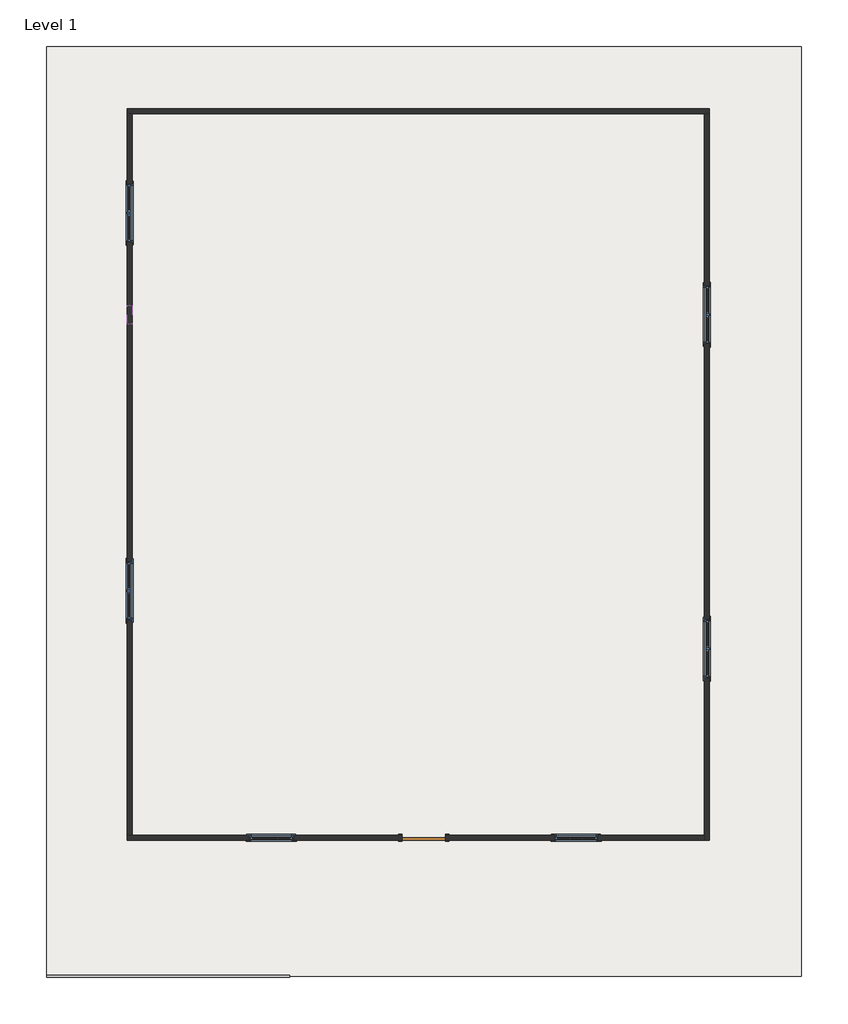
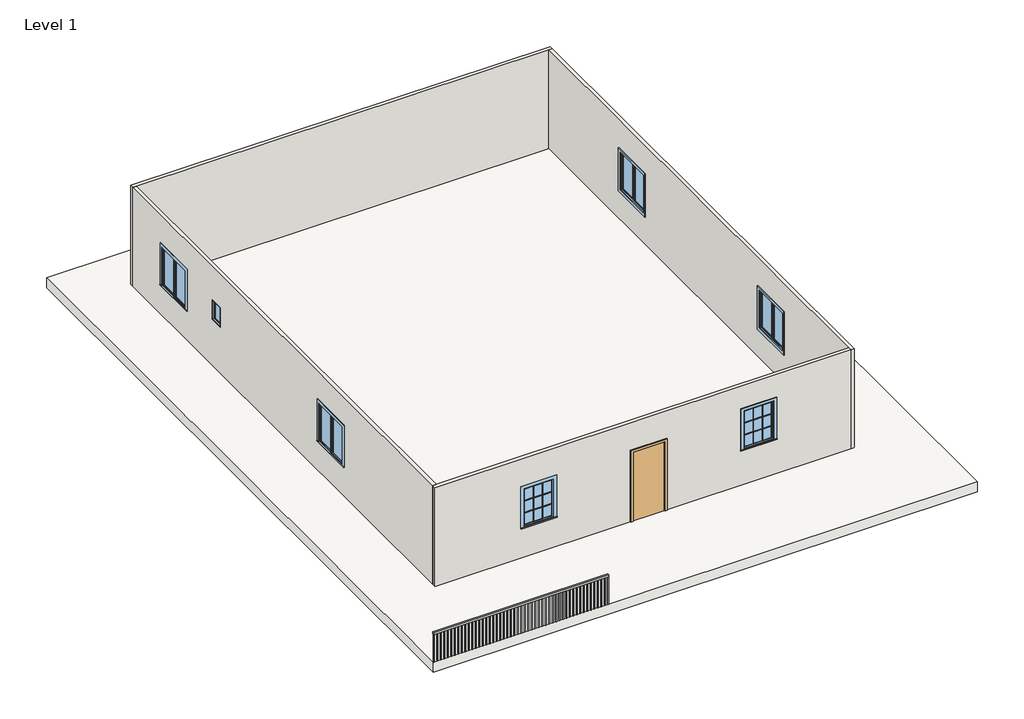
# One storey, incomplete: 7 windows, 4 walls, 1 door, 1 railing, 1 slab.
"""IFC4 building model written with IfcOpenShell, lengths in millimetres."""

from ifc_helpers import new_model, si_unit, frame, origin, origin_with_axes, place, context, project, spatial, polyline, outline, extrude, faceted_brep, transform, mapped, element, save
from components import door_048588e9, window_ad8769eb, window_90ef9153, window_a112695e

model = new_model("IFC4")

# Units and contexts
model_context = context("Model", 3, world=origin())
ifc_project = project(units=[si_unit("LENGTHUNIT", "METRE", prefix="MILLI")], contexts=[model_context])

# Site, building, storey
site = spatial("IfcSite", under=ifc_project)
building = spatial("IfcBuilding", under=site)
storey = spatial("IfcBuildingStorey", under=building, Name="Level 1", Elevation=0.0)

# Door
placement = place(None, origin())
door_shape = door_048588e9(model_context)
element("IfcDoor", 1, ObjectType="Single-Flush : 36\" x 84\"", at=placement, inside=storey, context=model_context, shape_type="MappedRepresentation", body=[
    mapped(door_shape, transform((7992.9168112, -1990.8718204, 0.0), x_axis=(-1.0, 0.0, 0.0), y_axis=(0.0, -1.0, 0.0), z_axis=(0.0, 0.0, 1.0))),
])

# Railing
element("IfcRailing", 2, ObjectType="Handrail - Rectangular", at=placement, inside=storey, context=model_context, shape_type="SweptSolid", body=[
    extrude(outline(polyline([(5173.5168112, -4873.0399729), (5173.5168112, -4923.8399729), (74.1689082, -4923.8399729), (74.1689082, -4873.0399729), (5173.5168112, -4873.0399729)])), frame((0.0, 0.0, 863.6), z_axis=(0.0, 0.0, 1.0), x_axis=(1.0, 0.0, 0.0)), (0.0, 0.0, 1.0), 50.8),
    extrude(outline(polyline([(103.0418112, -4888.9149729), (103.0418112, -4907.9649729), (83.9918112, -4907.9649729), (83.9918112, -4888.9149729), (103.0418112, -4888.9149729)])), origin_with_axes(), (0.0, 0.0, 1.0), 863.6),
    extrude(outline(polyline([(204.6418112, -4888.9149729), (204.6418112, -4907.9649729), (185.5918112, -4907.9649729), (185.5918112, -4888.9149729), (204.6418112, -4888.9149729)])), origin_with_axes(), (0.0, 0.0, 1.0), 863.6),
    extrude(outline(polyline([(306.2418112, -4888.9149729), (306.2418112, -4907.9649729), (287.1918112, -4907.9649729), (287.1918112, -4888.9149729), (306.2418112, -4888.9149729)])), origin_with_axes(), (0.0, 0.0, 1.0), 863.6),
    extrude(outline(polyline([(407.8418112, -4888.9149729), (407.8418112, -4907.9649729), (388.7918112, -4907.9649729), (388.7918112, -4888.9149729), (407.8418112, -4888.9149729)])), origin_with_axes(), (0.0, 0.0, 1.0), 863.6),
    extrude(outline(polyline([(509.4418112, -4888.9149729), (509.4418112, -4907.9649729), (490.3918112, -4907.9649729), (490.3918112, -4888.9149729), (509.4418112, -4888.9149729)])), origin_with_axes(), (0.0, 0.0, 1.0), 863.6),
    extrude(outline(polyline([(611.0418112, -4888.9149729), (611.0418112, -4907.9649729), (591.9918112, -4907.9649729), (591.9918112, -4888.9149729), (611.0418112, -4888.9149729)])), origin_with_axes(), (0.0, 0.0, 1.0), 863.6),
    extrude(outline(polyline([(712.6418112, -4888.9149729), (712.6418112, -4907.9649729), (693.5918112, -4907.9649729), (693.5918112, -4888.9149729), (712.6418112, -4888.9149729)])), origin_with_axes(), (0.0, 0.0, 1.0), 863.6),
    extrude(outline(polyline([(814.2418112, -4888.9149729), (814.2418112, -4907.9649729), (795.1918112, -4907.9649729), (795.1918112, -4888.9149729), (814.2418112, -4888.9149729)])), origin_with_axes(), (0.0, 0.0, 1.0), 863.6),
    extrude(outline(polyline([(915.8418112, -4888.9149729), (915.8418112, -4907.9649729), (896.7918112, -4907.9649729), (896.7918112, -4888.9149729), (915.8418112, -4888.9149729)])), origin_with_axes(), (0.0, 0.0, 1.0), 863.6),
    extrude(outline(polyline([(1017.4418112, -4888.9149729), (1017.4418112, -4907.9649729), (998.3918112, -4907.9649729), (998.3918112, -4888.9149729), (1017.4418112, -4888.9149729)])), origin_with_axes(), (0.0, 0.0, 1.0), 863.6),
    extrude(outline(polyline([(1119.0418112, -4888.9149729), (1119.0418112, -4907.9649729), (1099.9918112, -4907.9649729), (1099.9918112, -4888.9149729), (1119.0418112, -4888.9149729)])), origin_with_axes(), (0.0, 0.0, 1.0), 863.6),
    extrude(outline(polyline([(1220.6418112, -4888.9149729), (1220.6418112, -4907.9649729), (1201.5918112, -4907.9649729), (1201.5918112, -4888.9149729), (1220.6418112, -4888.9149729)])), origin_with_axes(), (0.0, 0.0, 1.0), 863.6),
    extrude(outline(polyline([(1322.2418112, -4888.9149729), (1322.2418112, -4907.9649729), (1303.1918112, -4907.9649729), (1303.1918112, -4888.9149729), (1322.2418112, -4888.9149729)])), origin_with_axes(), (0.0, 0.0, 1.0), 863.6),
    extrude(outline(polyline([(1423.8418112, -4888.9149729), (1423.8418112, -4907.9649729), (1404.7918112, -4907.9649729), (1404.7918112, -4888.9149729), (1423.8418112, -4888.9149729)])), origin_with_axes(), (0.0, 0.0, 1.0), 863.6),
    extrude(outline(polyline([(1525.4418112, -4888.9149729), (1525.4418112, -4907.9649729), (1506.3918112, -4907.9649729), (1506.3918112, -4888.9149729), (1525.4418112, -4888.9149729)])), origin_with_axes(), (0.0, 0.0, 1.0), 863.6),
    extrude(outline(polyline([(1627.0418112, -4888.9149729), (1627.0418112, -4907.9649729), (1607.9918112, -4907.9649729), (1607.9918112, -4888.9149729), (1627.0418112, -4888.9149729)])), origin_with_axes(), (0.0, 0.0, 1.0), 863.6),
    extrude(outline(polyline([(1728.6418112, -4888.9149729), (1728.6418112, -4907.9649729), (1709.5918112, -4907.9649729), (1709.5918112, -4888.9149729), (1728.6418112, -4888.9149729)])), origin_with_axes(), (0.0, 0.0, 1.0), 863.6),
    extrude(outline(polyline([(1830.2418112, -4888.9149729), (1830.2418112, -4907.9649729), (1811.1918112, -4907.9649729), (1811.1918112, -4888.9149729), (1830.2418112, -4888.9149729)])), origin_with_axes(), (0.0, 0.0, 1.0), 863.6),
    extrude(outline(polyline([(1931.8418112, -4888.9149729), (1931.8418112, -4907.9649729), (1912.7918112, -4907.9649729), (1912.7918112, -4888.9149729), (1931.8418112, -4888.9149729)])), origin_with_axes(), (0.0, 0.0, 1.0), 863.6),
    extrude(outline(polyline([(2033.4418112, -4888.9149729), (2033.4418112, -4907.9649729), (2014.3918112, -4907.9649729), (2014.3918112, -4888.9149729), (2033.4418112, -4888.9149729)])), origin_with_axes(), (0.0, 0.0, 1.0), 863.6),
    extrude(outline(polyline([(2135.0418112, -4888.9149729), (2135.0418112, -4907.9649729), (2115.9918112, -4907.9649729), (2115.9918112, -4888.9149729), (2135.0418112, -4888.9149729)])), origin_with_axes(), (0.0, 0.0, 1.0), 863.6),
    extrude(outline(polyline([(2236.6418112, -4888.9149729), (2236.6418112, -4907.9649729), (2217.5918112, -4907.9649729), (2217.5918112, -4888.9149729), (2236.6418112, -4888.9149729)])), origin_with_axes(), (0.0, 0.0, 1.0), 863.6),
    extrude(outline(polyline([(2338.2418112, -4888.9149729), (2338.2418112, -4907.9649729), (2319.1918112, -4907.9649729), (2319.1918112, -4888.9149729), (2338.2418112, -4888.9149729)])), origin_with_axes(), (0.0, 0.0, 1.0), 863.6),
    extrude(outline(polyline([(2439.8418112, -4888.9149729), (2439.8418112, -4907.9649729), (2420.7918112, -4907.9649729), (2420.7918112, -4888.9149729), (2439.8418112, -4888.9149729)])), origin_with_axes(), (0.0, 0.0, 1.0), 863.6),
    extrude(outline(polyline([(2541.4418112, -4888.9149729), (2541.4418112, -4907.9649729), (2522.3918112, -4907.9649729), (2522.3918112, -4888.9149729), (2541.4418112, -4888.9149729)])), origin_with_axes(), (0.0, 0.0, 1.0), 863.6),
    extrude(outline(polyline([(2643.0418112, -4888.9149729), (2643.0418112, -4907.9649729), (2623.9918112, -4907.9649729), (2623.9918112, -4888.9149729), (2643.0418112, -4888.9149729)])), origin_with_axes(), (0.0, 0.0, 1.0), 863.6),
    extrude(outline(polyline([(2744.6418112, -4888.9149729), (2744.6418112, -4907.9649729), (2725.5918112, -4907.9649729), (2725.5918112, -4888.9149729), (2744.6418112, -4888.9149729)])), origin_with_axes(), (0.0, 0.0, 1.0), 863.6),
    extrude(outline(polyline([(2846.2418112, -4888.9149729), (2846.2418112, -4907.9649729), (2827.1918112, -4907.9649729), (2827.1918112, -4888.9149729), (2846.2418112, -4888.9149729)])), origin_with_axes(), (0.0, 0.0, 1.0), 863.6),
    extrude(outline(polyline([(2947.8418112, -4888.9149729), (2947.8418112, -4907.9649729), (2928.7918112, -4907.9649729), (2928.7918112, -4888.9149729), (2947.8418112, -4888.9149729)])), origin_with_axes(), (0.0, 0.0, 1.0), 863.6),
    extrude(outline(polyline([(3049.4418112, -4888.9149729), (3049.4418112, -4907.9649729), (3030.3918112, -4907.9649729), (3030.3918112, -4888.9149729), (3049.4418112, -4888.9149729)])), origin_with_axes(), (0.0, 0.0, 1.0), 863.6),
    extrude(outline(polyline([(3151.0418112, -4888.9149729), (3151.0418112, -4907.9649729), (3131.9918112, -4907.9649729), (3131.9918112, -4888.9149729), (3151.0418112, -4888.9149729)])), origin_with_axes(), (0.0, 0.0, 1.0), 863.6),
    extrude(outline(polyline([(3252.6418112, -4888.9149729), (3252.6418112, -4907.9649729), (3233.5918112, -4907.9649729), (3233.5918112, -4888.9149729), (3252.6418112, -4888.9149729)])), origin_with_axes(), (0.0, 0.0, 1.0), 863.6),
    extrude(outline(polyline([(3354.2418112, -4888.9149729), (3354.2418112, -4907.9649729), (3335.1918112, -4907.9649729), (3335.1918112, -4888.9149729), (3354.2418112, -4888.9149729)])), origin_with_axes(), (0.0, 0.0, 1.0), 863.6),
    extrude(outline(polyline([(3455.8418112, -4888.9149729), (3455.8418112, -4907.9649729), (3436.7918112, -4907.9649729), (3436.7918112, -4888.9149729), (3455.8418112, -4888.9149729)])), origin_with_axes(), (0.0, 0.0, 1.0), 863.6),
    extrude(outline(polyline([(3557.4418112, -4888.9149729), (3557.4418112, -4907.9649729), (3538.3918112, -4907.9649729), (3538.3918112, -4888.9149729), (3557.4418112, -4888.9149729)])), origin_with_axes(), (0.0, 0.0, 1.0), 863.6),
    extrude(outline(polyline([(3659.0418112, -4888.9149729), (3659.0418112, -4907.9649729), (3639.9918112, -4907.9649729), (3639.9918112, -4888.9149729), (3659.0418112, -4888.9149729)])), origin_with_axes(), (0.0, 0.0, 1.0), 863.6),
    extrude(outline(polyline([(3760.6418112, -4888.9149729), (3760.6418112, -4907.9649729), (3741.5918112, -4907.9649729), (3741.5918112, -4888.9149729), (3760.6418112, -4888.9149729)])), origin_with_axes(), (0.0, 0.0, 1.0), 863.6),
    extrude(outline(polyline([(3862.2418112, -4888.9149729), (3862.2418112, -4907.9649729), (3843.1918112, -4907.9649729), (3843.1918112, -4888.9149729), (3862.2418112, -4888.9149729)])), origin_with_axes(), (0.0, 0.0, 1.0), 863.6),
    extrude(outline(polyline([(3963.8418112, -4888.9149729), (3963.8418112, -4907.9649729), (3944.7918112, -4907.9649729), (3944.7918112, -4888.9149729), (3963.8418112, -4888.9149729)])), origin_with_axes(), (0.0, 0.0, 1.0), 863.6),
    extrude(outline(polyline([(4065.4418112, -4888.9149729), (4065.4418112, -4907.9649729), (4046.3918112, -4907.9649729), (4046.3918112, -4888.9149729), (4065.4418112, -4888.9149729)])), origin_with_axes(), (0.0, 0.0, 1.0), 863.6),
    extrude(outline(polyline([(4167.0418112, -4888.9149729), (4167.0418112, -4907.9649729), (4147.9918112, -4907.9649729), (4147.9918112, -4888.9149729), (4167.0418112, -4888.9149729)])), origin_with_axes(), (0.0, 0.0, 1.0), 863.6),
    extrude(outline(polyline([(4268.6418112, -4888.9149729), (4268.6418112, -4907.9649729), (4249.5918112, -4907.9649729), (4249.5918112, -4888.9149729), (4268.6418112, -4888.9149729)])), origin_with_axes(), (0.0, 0.0, 1.0), 863.6),
    extrude(outline(polyline([(4370.2418112, -4888.9149729), (4370.2418112, -4907.9649729), (4351.1918112, -4907.9649729), (4351.1918112, -4888.9149729), (4370.2418112, -4888.9149729)])), origin_with_axes(), (0.0, 0.0, 1.0), 863.6),
    extrude(outline(polyline([(4471.8418112, -4888.9149729), (4471.8418112, -4907.9649729), (4452.7918112, -4907.9649729), (4452.7918112, -4888.9149729), (4471.8418112, -4888.9149729)])), origin_with_axes(), (0.0, 0.0, 1.0), 863.6),
    extrude(outline(polyline([(4573.4418112, -4888.9149729), (4573.4418112, -4907.9649729), (4554.3918112, -4907.9649729), (4554.3918112, -4888.9149729), (4573.4418112, -4888.9149729)])), origin_with_axes(), (0.0, 0.0, 1.0), 863.6),
    extrude(outline(polyline([(4675.0418112, -4888.9149729), (4675.0418112, -4907.9649729), (4655.9918112, -4907.9649729), (4655.9918112, -4888.9149729), (4675.0418112, -4888.9149729)])), origin_with_axes(), (0.0, 0.0, 1.0), 863.6),
    extrude(outline(polyline([(4776.6418112, -4888.9149729), (4776.6418112, -4907.9649729), (4757.5918112, -4907.9649729), (4757.5918112, -4888.9149729), (4776.6418112, -4888.9149729)])), origin_with_axes(), (0.0, 0.0, 1.0), 863.6),
    extrude(outline(polyline([(4878.2418112, -4888.9149729), (4878.2418112, -4907.9649729), (4859.1918112, -4907.9649729), (4859.1918112, -4888.9149729), (4878.2418112, -4888.9149729)])), origin_with_axes(), (0.0, 0.0, 1.0), 863.6),
    extrude(outline(polyline([(4979.8418112, -4888.9149729), (4979.8418112, -4907.9649729), (4960.7918112, -4907.9649729), (4960.7918112, -4888.9149729), (4979.8418112, -4888.9149729)])), origin_with_axes(), (0.0, 0.0, 1.0), 863.6),
    extrude(outline(polyline([(5081.4418112, -4888.9149729), (5081.4418112, -4907.9649729), (5062.3918112, -4907.9649729), (5062.3918112, -4888.9149729), (5081.4418112, -4888.9149729)])), origin_with_axes(), (0.0, 0.0, 1.0), 863.6),
    extrude(outline(polyline([(93.2189082, -4888.9149729), (93.2189082, -4907.9649729), (74.1689082, -4907.9649729), (74.1689082, -4888.9149729), (93.2189082, -4888.9149729)])), origin_with_axes(), (0.0, 0.0, 1.0), 863.6),
    extrude(outline(polyline([(5173.5168112, -4888.9149729), (5173.5168112, -4907.9649729), (5154.4668112, -4907.9649729), (5154.4668112, -4888.9149729), (5173.5168112, -4888.9149729)])), origin_with_axes(), (0.0, 0.0, 1.0), 863.6),
])

# Slab
element("IfcSlab", 3, ObjectType="Generic - 12\"", at=placement, inside=storey, context=model_context, shape_type="SweptSolid", body=[
    extrude(outline(polyline([(15923.7689082, 14608.7600271), (15923.7689082, -4898.4399729), (74.1689082, -4898.4399729), (74.1689082, 14608.7600271), (15923.7689082, 14608.7600271)])), frame((0.0, 0.0, -304.8), z_axis=(0.0, 0.0, 1.0), x_axis=(1.0, 0.0, 0.0)), (0.0, 0.0, 1.0), 304.8),
])

# Walls
element("IfcWall", 4, ObjectType="Generic - 4\" Brick", at=placement, inside=storey, context=model_context, shape_type="Brep", body=[
    faceted_brep([(1769.9168112, 13198.3281796, 0.0), (1871.5168112, 13198.3281796, 0.0), (13885.7168112, 13198.3281796, 0.0), (13987.3168112, 13198.3281796, 0.0), (13987.3168112, 13198.3281796, 3048.0), (13885.7168112, 13198.3281796, 3048.0), (1871.5168112, 13198.3281796, 3048.0), (1769.9168112, 13198.3281796, 3048.0), (1769.9168112, 13299.9281796, 0.0), (1769.9168112, 13299.9281796, 3048.0), (13987.3168112, 13299.9281796, 3048.0), (13987.3168112, 13299.9281796, 0.0)], [[[0, 1, 2, 3, 4, 5, 6, 7]], [[8, 9, 10, 11]], [[3, 2, 1, 0, 8, 11]], [[4, 3, 11, 10]], [[0, 7, 9, 8]], [[7, 6, 5, 4, 10, 9]]]),
])
element("IfcWall", 5, ObjectType="Generic - 4\" Brick", at=placement, inside=storey, context=model_context, shape_type="Brep", body=[
    faceted_brep([(13885.7168112, 13198.3281796, 0.0), (13885.7168112, -1940.0718204, 0.0), (13885.7168112, -2041.6718204, 0.0), (13885.7168112, -2041.6718204, 3048.0), (13885.7168112, -1940.0718204, 3048.0), (13885.7168112, 13198.3281796, 3048.0), (13885.7168112, 1361.9281796, 2133.6), (13885.7168112, 1361.9281796, 914.4), (13885.7168112, 2581.1281796, 914.4), (13885.7168112, 2581.1281796, 2133.6), (13885.7168112, 8372.3281796, 2133.6), (13885.7168112, 8372.3281796, 914.4), (13885.7168112, 9591.5281796, 914.4), (13885.7168112, 9591.5281796, 2133.6), (13987.3168112, 13198.3281796, 0.0), (13987.3168112, 13198.3281796, 3048.0), (13987.3168112, -2041.6718204, 3048.0), (13987.3168112, -2041.6718204, 0.0), (13987.3168112, 1361.9281796, 2133.6), (13987.3168112, 2581.1281796, 2133.6), (13987.3168112, 2581.1281796, 914.4), (13987.3168112, 1361.9281796, 914.4), (13987.3168112, 8372.3281796, 2133.6), (13987.3168112, 9591.5281796, 2133.6), (13987.3168112, 9591.5281796, 914.4), (13987.3168112, 8372.3281796, 914.4)], [[[0, 1, 2, 3, 4, 5], [6, 7, 8, 9], [10, 11, 12, 13]], [[14, 15, 16, 17], [18, 19, 20, 21], [22, 23, 24, 25]], [[2, 1, 0, 14, 17]], [[0, 5, 15, 14]], [[5, 4, 3, 16, 15]], [[3, 2, 17, 16]], [[7, 6, 18, 21]], [[8, 7, 21, 20]], [[9, 8, 20, 19]], [[6, 9, 19, 18]], [[11, 10, 22, 25]], [[12, 11, 25, 24]], [[13, 12, 24, 23]], [[10, 13, 23, 22]]]),
])
element("IfcWall", 6, ObjectType="Generic - 4\" Brick", at=placement, inside=storey, context=model_context, shape_type="Brep", body=[
    faceted_brep([(7535.7168112, -1940.0718204, 2133.6), (7535.7168112, -1940.0718204, 0.0), (1871.5168112, -1940.0718204, 0.0), (1769.9168112, -1940.0718204, 0.0), (1769.9168112, -1940.0718204, 3048.0), (1871.5168112, -1940.0718204, 3048.0), (13885.7168112, -1940.0718204, 3048.0), (13885.7168112, -1940.0718204, 0.0), (8450.1168112, -1940.0718204, 0.0), (8450.1168112, -1940.0718204, 2133.6), (10736.1168112, -1940.0718204, 2288.7570446), (10736.1168112, -1940.0718204, 1069.5570446), (11650.5168112, -1940.0718204, 1069.5570446), (11650.5168112, -1940.0718204, 2288.7570446), (4335.3168112, -1940.0718204, 2133.6), (4335.3168112, -1940.0718204, 914.4), (5249.7168112, -1940.0718204, 914.4), (5249.7168112, -1940.0718204, 2133.6), (1769.9168112, -2041.6718204, 0.0), (7535.7168112, -2041.6718204, 0.0), (7535.7168112, -2041.6718204, 2133.6), (8450.1168112, -2041.6718204, 2133.6), (8450.1168112, -2041.6718204, 0.0), (13885.7168112, -2041.6718204, 0.0), (13885.7168112, -2041.6718204, 3048.0), (1769.9168112, -2041.6718204, 3048.0), (10736.1168112, -2041.6718204, 2288.7570446), (11650.5168112, -2041.6718204, 2288.7570446), (11650.5168112, -2041.6718204, 1069.5570446), (10736.1168112, -2041.6718204, 1069.5570446), (4335.3168112, -2041.6718204, 2133.6), (5249.7168112, -2041.6718204, 2133.6), (5249.7168112, -2041.6718204, 914.4), (4335.3168112, -2041.6718204, 914.4)], [[[0, 1, 2, 3, 4, 5, 6, 7, 8, 9], [10, 11, 12, 13], [14, 15, 16, 17]], [[18, 19, 20, 21, 22, 23, 24, 25], [26, 27, 28, 29], [30, 31, 32, 33]], [[8, 7, 23, 22]], [[3, 2, 1, 19, 18]], [[6, 5, 4, 25, 24]], [[4, 3, 18, 25]], [[7, 6, 24, 23]], [[20, 19, 1, 0]], [[21, 20, 0, 9]], [[22, 21, 9, 8]], [[11, 10, 26, 29]], [[12, 11, 29, 28]], [[13, 12, 28, 27]], [[10, 13, 27, 26]], [[15, 14, 30, 33]], [[16, 15, 33, 32]], [[17, 16, 32, 31]], [[14, 17, 31, 30]]]),
])
element("IfcWall", 7, ObjectType="Generic - 4\" Brick", at=placement, inside=storey, context=model_context, shape_type="SweptSolid", body=[
    extrude(outline(polyline([(13198.3281796, 0.0), (-1940.0718204, 0.0), (-1940.0718204, 3048.0), (13198.3281796, 3048.0), (13198.3281796, 0.0)]), holes=[polyline([(8778.7281796, 2030.6539964), (8778.7281796, 1421.0539964), (9185.1281796, 1421.0539964), (9185.1281796, 2030.6539964), (8778.7281796, 2030.6539964)]), polyline([(11725.1281796, 914.4), (11725.1281796, 2133.6), (10505.9281796, 2133.6), (10505.9281796, 914.4), (11725.1281796, 914.4)]), polyline([(3800.3281796, 914.4), (3800.3281796, 2133.6), (2581.1281796, 2133.6), (2581.1281796, 914.4), (3800.3281796, 914.4)])]), frame((1769.9168112, 0.0, 0.0), z_axis=(1.0, 0.0, 0.0), x_axis=(0.0, 1.0, 0.0)), (0.0, 0.0, 1.0), 101.6),
])

# Windows
window_shape = window_ad8769eb(model_context)
element("IfcWindow", 8, ObjectType="Casement 3x3 with Trim : 36\" x 48\"", at=placement, inside=storey, context=model_context, shape_type="MappedRepresentation", body=[
    mapped(window_shape, transform((11193.3168112, -1990.8718204, 155.1570446), x_axis=(-1.0, 0.0, 0.0), y_axis=(0.0, -1.0, 0.0), z_axis=(0.0, 0.0, 1.0))),
])
element("IfcWindow", 9, ObjectType="Casement 3x3 with Trim : 36\" x 48\"", at=placement, inside=storey, context=model_context, shape_type="MappedRepresentation", body=[
    mapped(window_shape, transform((4792.5168112, -1990.8718204, 0.0), x_axis=(-1.0, 0.0, 0.0), y_axis=(0.0, -1.0, 0.0), z_axis=(0.0, 0.0, 1.0))),
])
window_2_shape = window_90ef9153(model_context)
element("IfcWindow", 10, ObjectType="Casement Dbl with Trim : 48\" x 48\"", at=placement, inside=storey, context=model_context, shape_type="MappedRepresentation", body=[
    mapped(window_2_shape, transform((1839.7668112, 11115.5281796, 0.0), x_axis=(0.0, 1.0, 0.0), y_axis=(-1.0, 0.0, 0.0), z_axis=(0.0, 0.0, 1.0))),
])
element("IfcWindow", 11, ObjectType="Casement Dbl with Trim : 48\" x 48\"", at=placement, inside=storey, context=model_context, shape_type="MappedRepresentation", body=[
    mapped(window_2_shape, transform((1839.7668112, 3190.7281796, 0.0), x_axis=(0.0, 1.0, 0.0), y_axis=(-1.0, 0.0, 0.0), z_axis=(0.0, 0.0, 1.0))),
])
element("IfcWindow", 12, ObjectType="Casement Dbl with Trim : 48\" x 48\"", at=placement, inside=storey, context=model_context, shape_type="MappedRepresentation", body=[
    mapped(window_2_shape, transform((13917.4668112, 1971.5281796, 0.0), x_axis=(0.0, -1.0, 0.0), y_axis=(1.0, 0.0, 0.0), z_axis=(0.0, 0.0, 1.0))),
])
element("IfcWindow", 13, ObjectType="Casement Dbl with Trim : 48\" x 48\"", at=placement, inside=storey, context=model_context, shape_type="MappedRepresentation", body=[
    mapped(window_2_shape, transform((13917.4668112, 8981.9281796, 0.0), x_axis=(0.0, -1.0, 0.0), y_axis=(1.0, 0.0, 0.0), z_axis=(0.0, 0.0, 1.0))),
])
window_3_shape = window_a112695e(model_context)
element("IfcWindow", 14, ObjectType="Fixed : 16\" x 24\"", at=placement, inside=storey, context=model_context, shape_type="MappedRepresentation", body=[
    mapped(window_3_shape, transform((1820.7168112, 8943.8281796, 506.6539964), x_axis=(0.0, -1.0, 0.0), y_axis=(1.0, 0.0, 0.0), z_axis=(0.0, 0.0, 1.0))),
])

save(model, "model.ifc")

# Revit data of these elements
# Type "Single-Flush : 36\" x 84\""
#   Type Mark = "1"
#   Construction Type Id = "MDOOR"
#   Assembly Code = "C1020"
#   Analytic Construction = "Metal"
#   Thickness = 0' - 2"
#   Heat Transfer Coefficient (U) = 0.651978 BTU/(h·ft²·°F)
#   Height = 7' - 0"
#   Trim Projection Ext = 0' - 1"
#   Trim Projection Int = 0' - 1"
#   Trim Width = 0' - 3"
#   Width = 3' - 0"
#   Define Thermal Properties by = 1
#   Door Material = Door - Panel
#   Frame Material = Door - Frame
#   Visual Light Transmittance = 0
#   Solar Heat Gain Coefficient = 0
#   Function = (empty or 0)
#   Wall Closure = (empty or 0)
# Type "Handrail - Rectangular"
#   Assembly Code = "C2010400"
#   built-in parameter 1008612 = 0.0416667 (stored number, unit not read)
#   built-in parameter 1008611 = 0.0416667 (stored number, unit not read)
#   built-in parameter 1008609 = 0.333333 (stored number, unit not read)
#   built-in parameter 1008604 = 0.166667 (stored number, unit not read)
#   built-in parameter 1008603 = 0.166667 (stored number, unit not read)
#   Railing Height = 3' - 0"
#   built-in parameter 1008630 = 2
#   built-in parameter 1008610 = 2
#   built-in parameter 1008618 = Baluster - Square : 3/4"
# Type "Generic - 12\""
#   Assembly Code = "B1010"
#   Function = 0
#   Layers, outside or top first: 1' - 0" no material (function 1)
# Type "Generic - 4\" Brick"
#   Assembly Code = "B2010"
#   Layers, outside or top first: 0' - 4" "Brick, Common" (function 1)
# Type "Casement 3x3 with Trim : 36\" x 48\""
#   Type Mark = "10"
#   Construction Type Id = "GSP4R"
#   Assembly Code = "B2020100"
#   Analytic Construction = "1/8 in Pilkington single glazing"
#   Visual Light Transmittance = 0.9
#   Solar Heat Gain Coefficient = 0.78
#   Heat Transfer Coefficient (U) = 0.6496 BTU/(h·ft²·°F)
#   Height = 4' - 0"
#   Default Sill Height = 3' - 0"
#   Trim Projection - Ext. = 0' - 0 1/2"
#   Trim Projection - Int. = 0' - 0 3/4"
#   Trim Width - Exterior = 0' - 3 1/2"
#   Trim Width - Interior = 0' - 3 1/2"
#   Width = 3' - 0"
#   Window Inset = 0' - 0 3/4"
#   Define Thermal Properties by = 1
#   Glass Pane Material = Glass
#   Sash Material = Sash
#   Trim Exterior Material = Trim
#   Trim Interior Material = Trim
#   Wall Closure = (empty or 0)
# Type "Casement Dbl with Trim : 48\" x 48\""
#   Type Mark = "13"
#   Construction Type Id = "GSP4R"
#   Assembly Code = "B2020100"
#   Analytic Construction = "1/8 in Pilkington single glazing"
#   Visual Light Transmittance = 0.9
#   Solar Heat Gain Coefficient = 0.78
#   Heat Transfer Coefficient (U) = 0.6496 BTU/(h·ft²·°F)
#   Height = 4' - 0"
#   Default Sill Height = 3' - 0"
#   Trim Projection - Ext. = 0' - 0 1/2"
#   Trim Projection - Int. = 0' - 0 3/4"
#   Trim Width - Exterior = 0' - 3 1/2"
#   Trim Width - Interior = 0' - 3 1/2"
#   Width = 4' - 0"
#   Window Inset = 0' - 0 3/4"
#   Define Thermal Properties by = 1
#   Glass Pane Material = Glass
#   Sash Material = Sash
#   Trim Exterior Material = Trim
#   Trim Interior Material = Trim
#   Wall Closure = (empty or 0)
# Type "Fixed : 16\" x 24\""
#   Type Mark = "4"
#   Construction Type Id = "GSP4R"
#   Assembly Code = "B2020100"
#   Analytic Construction = "1/8 in Pilkington single glazing"
#   Visual Light Transmittance = 0.9
#   Solar Heat Gain Coefficient = 0.78
#   Heat Transfer Coefficient (U) = 0.6496 BTU/(h·ft²·°F)
#   Height = 2' - 0"
#   Default Sill Height = 3' - 0"
#   Width = 1' - 4"
#   Window Inset = 0' - 0 3/4"
#   Define Thermal Properties by = 1
#   Glass Pane Material = Glass
#   Sash Material = Sash
#   Wall Closure = (empty or 0)
# Element 1 (IfcDoor, "Single-Flush : 36\" x 84\"")
#   Phase Created = New Construction
#   Materials on its faces: "Door - Frame", "Door - Panel"
# Element 2 (IfcRailing, "Handrail - Rectangular")
#   Phase Created = New Construction
# Element 3 (IfcSlab, "Generic - 12\"")
#   Height Offset From Level = 0' - 0"
#   Phase Created = New Construction
#   Materials on its faces: "Default Floor"
# Elements 4, 5, 6, 7 (IfcWall, "Generic - 4\" Brick")
#   Top Offset = 0' - 0"
#   Base Offset = 0' - 0"
#   Unconnected Height = 10' - 0"
#   wall height = 10' - 0"
#   Phase Created = New Construction
#   Base Constraint = Level 1
#   Materials on its faces: "Brick, Common"
# Element 8 (IfcWindow, "Casement 3x3 with Trim : 36\" x 48\"")
#   Mark = "13"
#   Phase Created = New Construction
#   Materials on its faces: "Sash", "Glass", "Trim"
# Element 9 (IfcWindow, "Casement 3x3 with Trim : 36\" x 48\"")
#   Mark = "14"
#   Phase Created = New Construction
#   Materials on its faces: "Sash", "Glass", "Trim"
# Element 10 (IfcWindow, "Casement Dbl with Trim : 48\" x 48\"")
#   Mark = "21"
#   Phase Created = New Construction
#   Materials on its faces: "Sash", "Trim", "Glass"
# Element 11 (IfcWindow, "Casement Dbl with Trim : 48\" x 48\"")
#   Mark = "22"
#   Phase Created = New Construction
#   Materials on its faces: "Sash", "Trim", "Glass"
# Element 12 (IfcWindow, "Casement Dbl with Trim : 48\" x 48\"")
#   Mark = "28"
#   Phase Created = New Construction
#   Materials on its faces: "Sash", "Trim", "Glass"
# Element 13 (IfcWindow, "Casement Dbl with Trim : 48\" x 48\"")
#   Mark = "30"
#   Phase Created = New Construction
#   Materials on its faces: "Sash", "Trim", "Glass"
# Element 14 (IfcWindow, "Fixed : 16\" x 24\"")
#   Mark = "2"
#   Phase Created = New Construction
#   Materials on its faces: "Sash", "Glass"
# Materials
#   "Door - Panel": class "Wood", colour RGB 210 159 95, transparency 0
#   "Door - Frame": colour RGB 118 70 51, transparency 0
#   "Brick, Common": class "Masonry", colour RGB 170 98 104, transparency 0, Description = "Common brick", Cost = 0
#   "Glass": class "Glass", colour RGB 0 128 192, transparency 0.75, Description = "Soda Lime Glass", Cost = 0
#   "Sash": class "Wood", colour RGB 224 178 126, transparency 0
#   "Trim": class "Wood", colour RGB 224 178 126, transparency 0
#   "Default Floor": colour RGB 128 128 128, transparency 0
